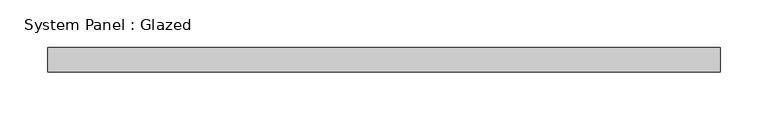
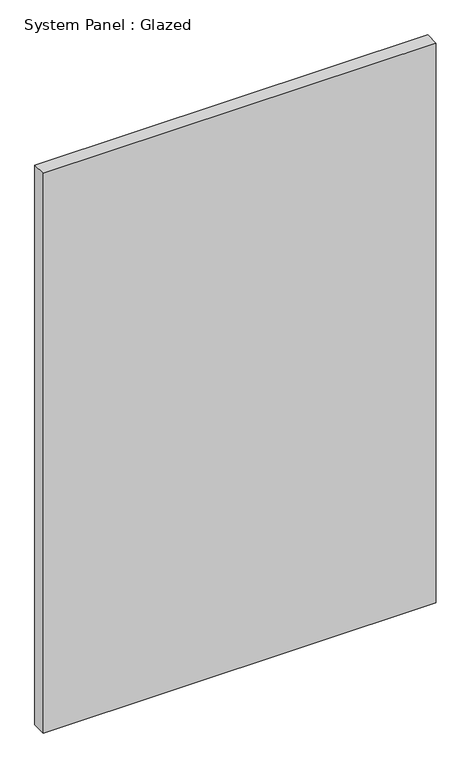
"""IFC4 building model written with IfcOpenShell, lengths in millimetres: plate geometry, System Panel : Glazed."""

from ifc_helpers import new_model, si_unit, origin, origin_with_axes, place, context, project, spatial, polyline, outline, extrude, source, transform, mapped, element, save


def system_panel_glazed_fc79919b(model_context):
    return source(origin(), model_context, "Body", "SweptSolid", [
        extrude(outline(polyline([(350.3083333, 19.05), (-350.3083333, 19.05), (-350.3083333, 44.45), (350.3083333, 44.45), (350.3083333, 19.05)])), origin_with_axes(), (0.0, 0.0, 1.0), 1054.1),
    ])


if __name__ == "__main__":
    model = new_model("IFC4")
    model_context = context("Model", 3, world=origin())
    ifc_project = project(units=[si_unit("LENGTHUNIT", "METRE", prefix="MILLI")], contexts=[model_context])
    site = spatial("IfcSite", under=ifc_project)
    building = spatial("IfcBuilding", under=site)
    placement = place(None, origin())
    system_panel_glazed_shape = system_panel_glazed_fc79919b(model_context)
    element("IfcPlate", 1, ObjectType="System Panel : Glazed", at=placement, inside=building, context=model_context, shape_type="MappedRepresentation", body=[
        mapped(system_panel_glazed_shape, transform((0.0, 0.0, 0.0), x_axis=(1.0, 0.0, 0.0), y_axis=(0.0, 1.0, 0.0), z_axis=(0.0, 0.0, 1.0))),
    ])
    save(model, "model.ifc")

# Revit data of these elements
# Type "System Panel : Glazed"
#   Construction Type Id = "GSP4R"
#   Analytic Construction = "1/8 in Pilkington single glazing"
#   Visual Light Transmittance = 0.9
#   Solar Heat Gain Coefficient = 0.86
#   Heat Transfer Coefficient (U) = 1.18115 BTU/(h·ft²·°F)
# Element 1 (IfcPlate, "System Panel : Glazed")
#   Materials on its faces: "Glass"
# Materials
#   "Glass": class "Glass", colour RGB 0 128 192, transparency 0.75, Description = "Soda Lime Glass", Cost = 0
